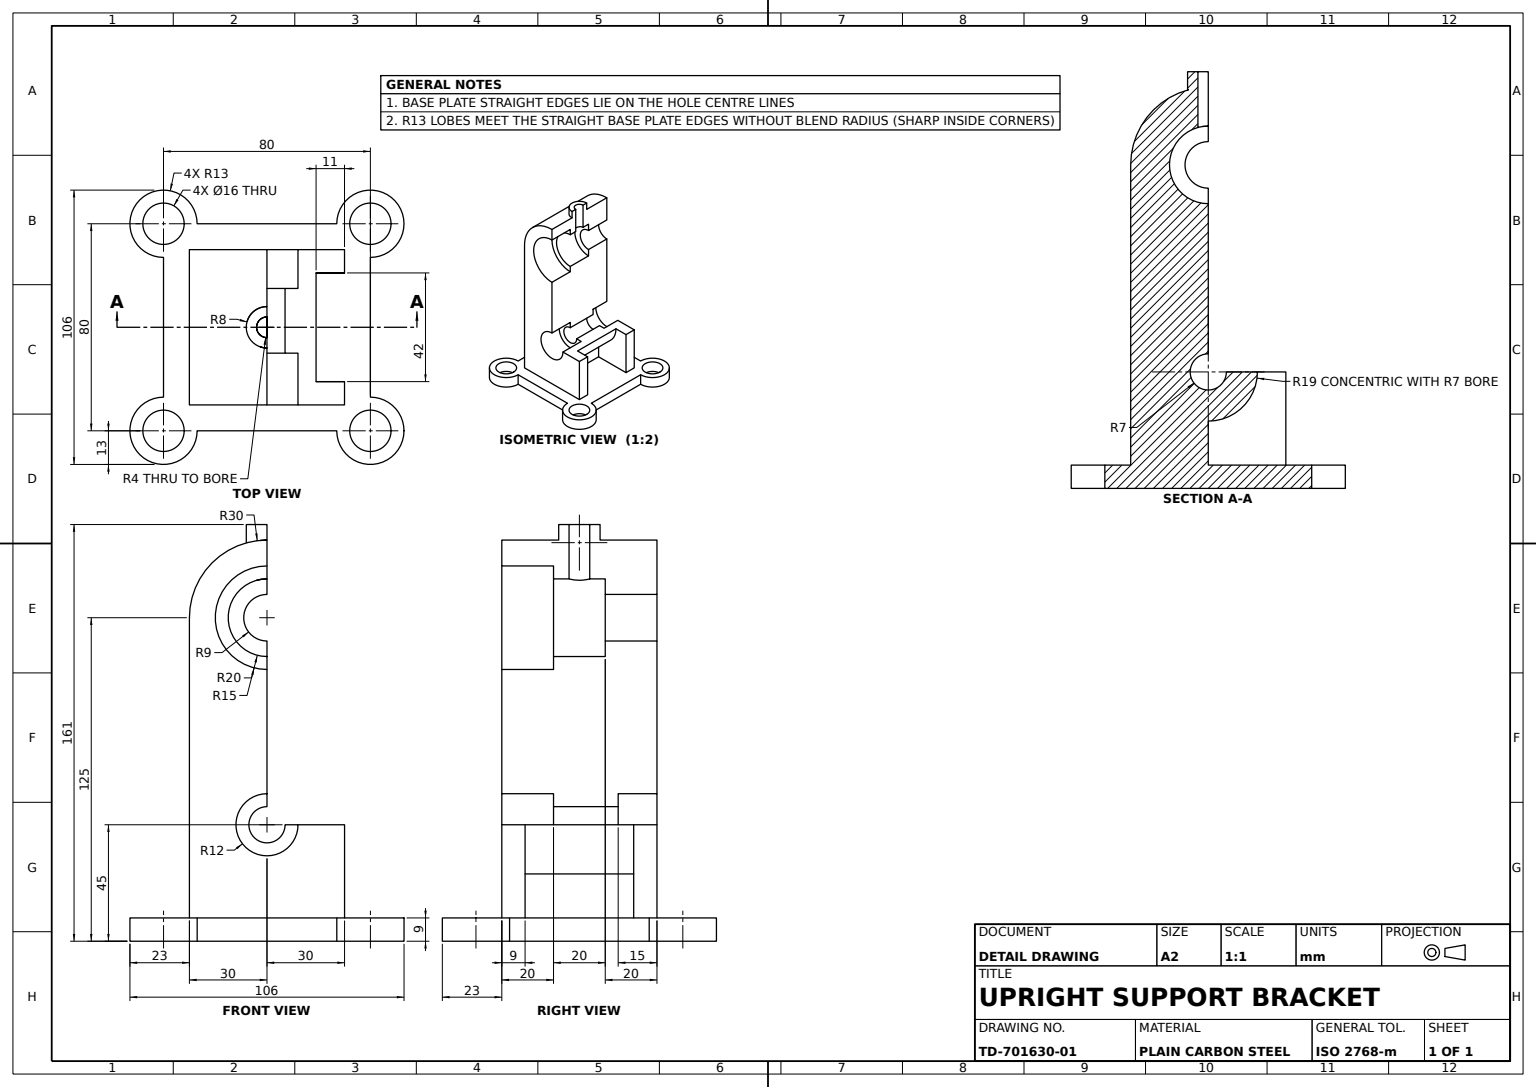
SolidWorks part; units mm, degrees
material "Plain Carbon Steel"
ref_plane "Front Plane" through (0, 0, 0) normal (0, 0, 1) x (1, 0, 0)
ref_plane "Top Plane" through (0, 0, 0) normal (0, 1, 0) x (1, 0, 0)
ref_plane "Right Plane" through (0, 0, 0) normal (1, 0, 0) x (0, 0, -1)
sketch "Base Flange Sketch" plane through (0, 0, 0) normal (0, 1, 0) x (1, 0, 0)
  line L0 (-27, 40) -> (27, 40)
  line L1 (0, 0) -> (134.5857, 0) construction
  line L2 (-27, -40) -> (27, -40)
  line L3 (-40, 27) -> (-40, -27)
  line L4 (0, 0) -> (0, 117.8529) construction
  line L5 (40, 27) -> (40, -27)
  arc A0 (-27, 40) -> (-40, 27) centre (-40, 40) ccw
  arc A1 (40, 27) -> (27, 40) centre (40, 40) ccw
  arc A2 (-40, -27) -> (-27, -40) centre (-40, -40) ccw
  arc A3 (27, -40) -> (40, -27) centre (40, -40) ccw
  circle A4 centre (-40, 40) radius 8
  circle A5 centre (40, 40) radius 8
  circle A6 centre (40, -40) radius 8
  circle A7 centre (-40, -40) radius 8
  dimension "D1" = 26
  dimension "D6" = 134.5857
  dimension "D4" = 16
  dimension "D2" = 80
  dimension "D3" = 80
  dimension "D5" = 2
  dimension "D7" = 117.8529
  dimension "D8" = 2
extrude "Base Flange" add sketch "Base Flange Sketch" along normal blind 9
sketch "Tower Profile Sketch" plane through (0, 0, 0) normal (1, 0, 0) x (0, 0, -1)
  line L0 (-30, 9) -> (-30, 125)
  line L1 (-27, 9) -> (27, 9) construction
  line L2 (0, 155) -> (0, 45)
  line L3 (0, 45) -> (30, 45)
  line L4 (30, 45) -> (30, 9)
  line L5 (30, 9) -> (-30, 9)
  arc A0 (-30, 125) -> (0, 155) centre (0, 125) cw
  dimension "D5" = 116
  dimension "D1" = 30
  dimension "D2" = 30
  dimension "D3" = 30
  dimension "D4" = 36
extrude "Tower" add sketch "Tower Profile Sketch" along normal mid plane 60
sketch "Bore Axis Sketch" plane through (30, 0, 0) normal (1, 0, 0) x (0, 0, -1)
  circle A0 centre (0, 125) radius 9
  dimension "D1" = 18
sketch "Lower Bore Profile Sketch" plane through (0, 0, 0) normal (0, 0, -1) x (-1, 0, 0)
  line L0 (-30, 125) -> (30, 125) construction
  line L1 (-30, 134) -> (-30, 116) construction
  line L2 (30, 45) -> (30, 155) construction
  line L3 (30, 134) -> (10, 134)
  line L4 (10, 134) -> (10, 140)
  line L5 (10, 140) -> (-10, 140)
  line L6 (-10, 140) -> (-10, 145)
  line L7 (-10, 145) -> (-30, 145)
  line L8 (-30, 45) -> (-30, 155) construction
  line L9 (-30, 145) -> (-30, 125)
  line L10 (-30, 125) -> (30, 125)
  line L11 (30, 125) -> (30, 134)
  dimension "D1" = 9
  dimension "D2" = 15
  dimension "D3" = 20
  dimension "D4" = 20
  dimension "D5" = 20
revolve "Lower Bore" cut sketch "Lower Bore Profile Sketch" angle 360 about L0
sketch "Upper Bore Profile Sketch" plane through (0, 0, 0) normal (0, 0, -1) x (-1, 0, 0)
  line L0 (30, 45) -> (-30, 45) construction
  line L1 (30, 57) -> (15, 57)
  line L2 (30, 45) -> (30, 116) construction
  line L3 (15, 57) -> (15, 52)
  line L4 (15, 52) -> (-10, 52)
  line L5 (-10, 52) -> (-10, 57)
  line L6 (-10, 57) -> (-30, 57)
  line L7 (-30, 45) -> (-30, 105) construction
  line L8 (-30, 57) -> (-30, 45)
  line L9 (-30, 45) -> (30, 45)
  line L10 (30, 45) -> (30, 57)
  dimension "D1" = 12
  dimension "D2" = 7
  dimension "D3" = 12
  dimension "D4" = 20
  dimension "D5" = 25
revolve "Upper Bore" cut sketch "Upper Bore Profile Sketch" angle 360 about L0
sketch "Side Slot Sketch" plane through (0, 0, 0) normal (1, 0, 0) x (0, 0, -1)
  line L0 (19, 45) -> (30, 45)
  line L1 (30, 45) -> (30, 9)
  line L2 (30, 9) -> (0, 9)
  line L3 (-30, 9) -> (30, 9) construction
  line L4 (0, 9) -> (0, 26)
  arc A0 (0, 26) -> (19, 45) centre (0, 45) ccw
  dimension "D1" = 38
extrude "Side Slot" cut sketch "Side Slot Sketch" against normal mid plane 42
ref_plane "Clip Boss Plane" through (0, 155, 0) normal (0, 1, 0) x (1, 0, 0)
sketch "Clip Boss Sketch" plane through (0, 155, 0) normal (0, 1, 0) x (1, 0, 0)
  line L0 (-8, 0) -> (8, 0) construction
  line L1 (-8, 0) -> (-4, 0)
  line L2 (4, 0) -> (8, 0)
  arc A0 (-8, 0) -> (8, 0) centre (0, 0) ccw
  arc A1 (-4, 0) -> (4, 0) centre (0, 0) ccw
  dimension "D1" = 16
  dimension "D2" = 8
extrude "Clip Boss" add sketch "Clip Boss Sketch" along normal blind 6 and the other way blind 1
sketch "Clip Slot Sketch" plane through (0, 155, 0) normal (0, 1, 0) x (1, 0, 0)
  line L0 (-4, 0) -> (4, 0)
  arc A0 (-4, 0) -> (4, 0) centre (0, 0) ccw
  dimension "D1" = 4
extrude "Clip Slot" cut sketch "Clip Slot Sketch" against normal up to surface (15 mm away)
